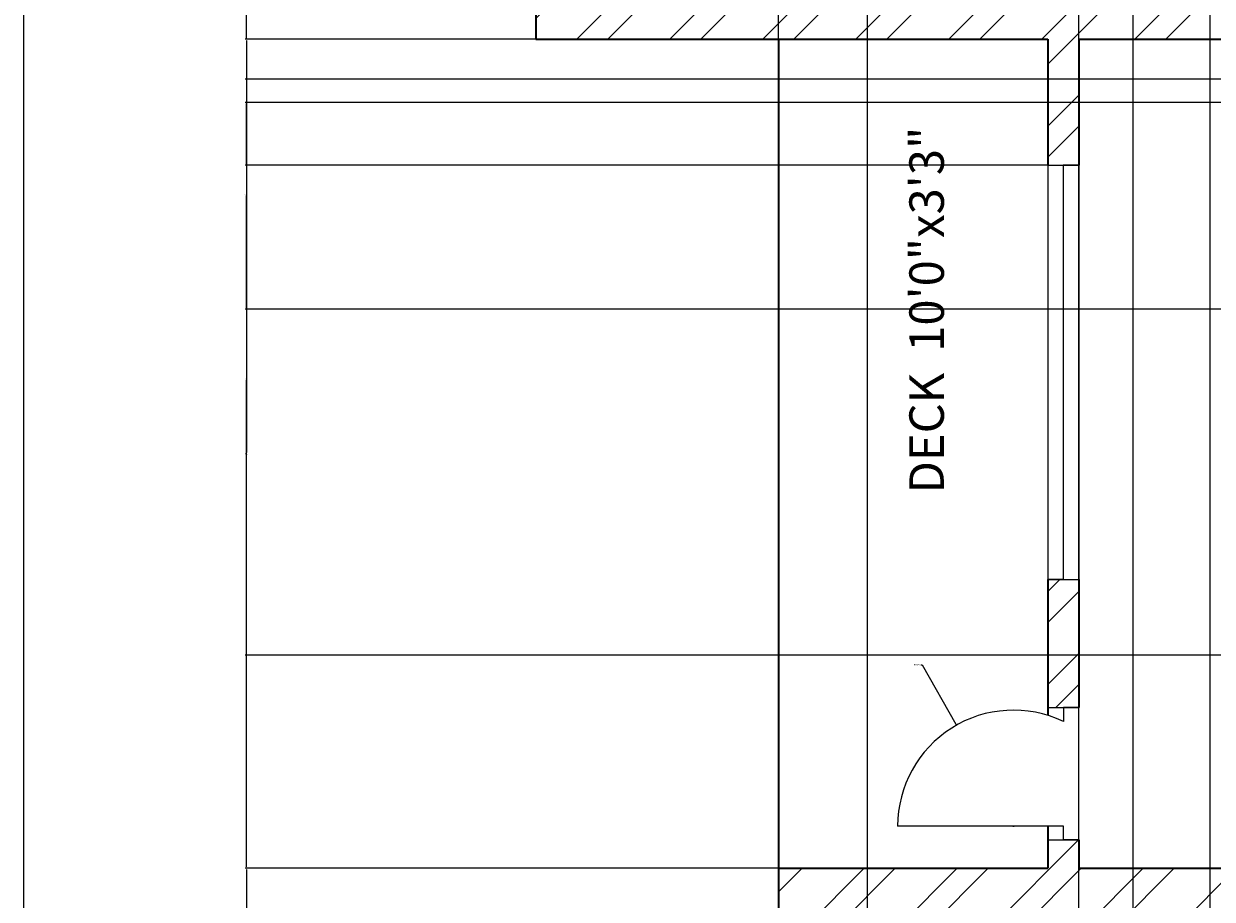
# Model space of a CAD drawing. Units: inches. Extents: x 1748 to 2382, y 1346 to 2284.
# Tile 7 of 26: x 1748 to 1920, y 1730 to 1857. Entities that reach past the tile are written whole.
import ezdxf

# ---------------------------------------------------------------- set-up
doc = ezdxf.new("R2010")
doc.units = ezdxf.units.IN
for name, color, linetype, lineweight in [('A-ANNO-DIMS', 2, 'Continuous', 18), ('A-ANNO-TTLB', 7, 'Continuous', 25), ('A-AREA-IDEN', 7, 'Continuous', 18), ('A-DOOR', 21, 'Continuous', 18), ('A-GLAZ', 191, 'Continuous', 18), ('A-WALL', 7, 'Continuous', 35), ('A-WALL-PATT', 9, 'Continuous', 13)]:
    doc.layers.add(name, color=color, linetype=linetype, lineweight=lineweight)
doc.styles.get("Standard").update_dxf_attribs({"font": 'arial.ttf'})
doc.dimstyles.get("Standard").update_dxf_attribs({"dimtxt": 0.18, "dimasz": 0.18, "dimexe": 0.18, "dimexo": 0.0625, "dimgap": 0.09, "dimtad": 0, "dimtih": 1, "dimtoh": 1, "dimdec": 4, "dimzin": 0, "dimdsep": 46, "dimtxsty": 'Standard', "dimcen": 0.09, "dimadec": 0, "dimazin": 0, "dimtfac": 1, "dimtdec": 4, "dimtofl": 0, "dimtmove": 0, "dimatfit": 3, "dimfxl": 1, "dimtolj": 1, "dimtzin": 0, "dimarcsym": 0})

# ---------------------------------------------------------------- blocks, each defined once
blk = doc.blocks.new('*D41')
at = {"layer": 'A-ANNO-DIMS', "color": 0, "lineweight": -2, "transparency": 16777216}
for p, q in [((1821.96, 1854.91), (1821.96, 2274.93)), ((1822.14, 2274.75), (1839.16, 2274.75)), ((1856.96, 2274.75), (1839.95, 2274.75)), ((1857.14, 1854.91), (1857.14, 2274.93))]:
    blk.add_line(p, q, dxfattribs=at)
at = {"layer": 'A-ANNO-DIMS', "color": 0, "transparency": 16777216}
for points in [[(1822.14, 2274.78), (1822.14, 2274.72), (1821.96, 2274.75)], [(1856.96, 2274.78), (1856.96, 2274.72), (1857.14, 2274.75)]]:
    blk.add_solid(points, dxfattribs=at)
at = {"layer": 'Defpoints', "color": 0, "transparency": 16777216}
for p in [(1857.14, 2274.75), (1821.96, 1854.85), (1857.14, 1854.85)]:
    blk.add_point(p, dxfattribs=at)
at = {"layer": 'A-ANNO-DIMS', "color": 0, "transparency": 16777216, "insert": (1839.55, 2274.75), "char_height": 0.18, "attachment_point": 5}
blk.add_mtext('\\A1;35.18', dxfattribs=at)
blk = doc.blocks.new('*D43')
at = {"layer": 'A-ANNO-DIMS', "color": 0, "lineweight": -2, "transparency": 16777216}
for p, q in [((1857.08, 1854.85), (1779.88, 1854.85)), ((1780.06, 1854.67), (1780.06, 1795.03)), ((1780.06, 1735.03), (1780.06, 1794.67)), ((1857.08, 1734.85), (1779.88, 1734.85))]:
    blk.add_line(p, q, dxfattribs=at)
at = {"layer": 'A-ANNO-DIMS', "color": 0, "transparency": 16777216}
for points in [[(1780.03, 1854.67), (1780.09, 1854.67), (1780.06, 1854.85)], [(1780.03, 1735.03), (1780.09, 1735.03), (1780.06, 1734.85)]]:
    blk.add_solid(points, dxfattribs=at)
at = {"layer": 'Defpoints', "color": 0, "transparency": 16777216}
for p in [(1780.06, 1854.85), (1857.14, 1854.85), (1857.14, 1734.85)]:
    blk.add_point(p, dxfattribs=at)
at = {"layer": 'A-ANNO-DIMS', "color": 0, "transparency": 16777216, "insert": (1780.06, 1794.85), "char_height": 0.18, "attachment_point": 5}
blk.add_mtext('\\A1;120', dxfattribs=at)
blk = doc.blocks.new('*D44')
at = {"layer": 'A-ANNO-DIMS', "color": 0, "lineweight": -2, "transparency": 16777216}
for p, q in [((1821.9, 1892.79), (1779.88, 1892.79)), ((1780.06, 1892.61), (1780.06, 1874)), ((1780.06, 1855.03), (1780.06, 1873.64)), ((1821.9, 1854.85), (1779.88, 1854.85))]:
    blk.add_line(p, q, dxfattribs=at)
at = {"layer": 'A-ANNO-DIMS', "color": 0, "transparency": 16777216}
for points in [[(1780.03, 1892.61), (1780.09, 1892.61), (1780.06, 1892.79)], [(1780.03, 1855.03), (1780.09, 1855.03), (1780.06, 1854.85)]]:
    blk.add_solid(points, dxfattribs=at)
at = {"layer": 'Defpoints', "color": 0, "transparency": 16777216}
for p in [(1780.06, 1892.79), (1821.96, 1892.79), (1821.96, 1854.85)]:
    blk.add_point(p, dxfattribs=at)
at = {"layer": 'A-ANNO-DIMS', "color": 0, "transparency": 16777216, "insert": (1780.06, 1873.82), "char_height": 0.18, "attachment_point": 5}
blk.add_mtext('\\A1;37.94', dxfattribs=at)
blk = doc.blocks.new('*D48')
at = {"layer": 'A-ANNO-DIMS', "color": 0, "lineweight": -2, "transparency": 16777216}
for p, q in [((2130.9, 1849.07), (1779.88, 1849.07)), ((1780.06, 1848.89), (1780.06, 1832.62)), ((1780.06, 1815.98), (1780.06, 1832.25)), ((2130.9, 1815.8), (1779.88, 1815.8))]:
    blk.add_line(p, q, dxfattribs=at)
at = {"layer": 'A-ANNO-DIMS', "color": 0, "transparency": 16777216}
for points in [[(1780.03, 1848.89), (1780.09, 1848.89), (1780.06, 1849.07)], [(1780.03, 1815.98), (1780.09, 1815.98), (1780.06, 1815.8)]]:
    blk.add_solid(points, dxfattribs=at)
at = {"layer": 'Defpoints', "color": 0, "transparency": 16777216}
for p in [(1780.06, 1849.07), (2130.96, 1849.07), (2130.96, 1815.8)]:
    blk.add_point(p, dxfattribs=at)
at = {"layer": 'A-ANNO-DIMS', "color": 0, "transparency": 16777216, "insert": (1780.06, 1832.43), "char_height": 0.18, "attachment_point": 5}
blk.add_mtext('\\A1;33.27', dxfattribs=at)
blk = doc.blocks.new('*D50')
at = {"layer": 'A-ANNO-DIMS', "color": 0, "lineweight": -2, "transparency": 16777216}
for p, q in [((1869.96, 2223.79), (1869.96, 1360.47)), ((1908.44, 2223.79), (1908.44, 1360.47)), ((1870.14, 1360.65), (1888.81, 1360.65)), ((1908.26, 1360.65), (1889.6, 1360.65))]:
    blk.add_line(p, q, dxfattribs=at)
at = {"layer": 'A-ANNO-DIMS', "color": 0, "transparency": 16777216}
for points in [[(1870.14, 1360.68), (1870.14, 1360.62), (1869.96, 1360.65)], [(1908.26, 1360.68), (1908.26, 1360.62), (1908.44, 1360.65)]]:
    blk.add_solid(points, dxfattribs=at)
at = {"layer": 'Defpoints', "color": 0, "transparency": 16777216}
for p in [(1869.96, 2223.85), (1908.44, 2223.85), (1908.44, 1360.65)]:
    blk.add_point(p, dxfattribs=at)
at = {"layer": 'A-ANNO-DIMS', "color": 0, "transparency": 16777216, "insert": (1889.2, 1360.65), "char_height": 0.18, "attachment_point": 5}
blk.add_mtext('\\A1;38.48', dxfattribs=at)
blk = doc.blocks.new('*D60')
at = {"layer": 'A-ANNO-DIMS', "color": 0, "lineweight": -2, "transparency": 16777216}
for p, q in [((2206.01, 1845.68), (1779.88, 1845.68)), ((1780.06, 1845.5), (1780.06, 1805.86)), ((1780.06, 1765.86), (1780.06, 1805.5)), ((2206.01, 1765.68), (1779.88, 1765.68))]:
    blk.add_line(p, q, dxfattribs=at)
at = {"layer": 'A-ANNO-DIMS', "color": 0, "transparency": 16777216}
for points in [[(1780.03, 1845.5), (1780.09, 1845.5), (1780.06, 1845.68)], [(1780.03, 1765.86), (1780.09, 1765.86), (1780.06, 1765.68)]]:
    blk.add_solid(points, dxfattribs=at)
at = {"layer": 'Defpoints', "color": 0, "transparency": 16777216}
for p in [(1780.06, 1845.68), (2206.07, 1845.68), (2206.07, 1765.68)]:
    blk.add_point(p, dxfattribs=at)
at = {"layer": 'A-ANNO-DIMS', "color": 0, "transparency": 16777216, "insert": (1780.06, 1805.68), "char_height": 0.18, "attachment_point": 5}
blk.add_mtext('\\A1;80', dxfattribs=at)
blk = doc.blocks.new('*D64')
at = {"layer": 'A-ANNO-DIMS', "color": 0, "lineweight": -2, "transparency": 16777216}
for p, q in [((1900.64, 1476.91), (1900.64, 2274.93)), ((1900.82, 2274.75), (1909.7, 2274.75)), ((1919.5, 2274.75), (1910.62, 2274.75)), ((1919.68, 1476.91), (1919.68, 2274.93))]:
    blk.add_line(p, q, dxfattribs=at)
at = {"layer": 'A-ANNO-DIMS', "color": 0, "transparency": 16777216}
for points in [[(1900.82, 2274.78), (1900.82, 2274.72), (1900.64, 2274.75)], [(1919.5, 2274.78), (1919.5, 2274.72), (1919.68, 2274.75)]]:
    blk.add_solid(points, dxfattribs=at)
at = {"layer": 'Defpoints', "color": 0, "transparency": 16777216}
for p in [(1919.68, 2274.75), (1900.64, 1476.85), (1919.68, 1476.85)]:
    blk.add_point(p, dxfattribs=at)
at = {"layer": 'A-ANNO-DIMS', "color": 0, "transparency": 16777216, "insert": (1910.16, 2274.75), "char_height": 0.18, "attachment_point": 5}
blk.add_mtext('\\A1;19.035', dxfattribs=at)
blk = doc.blocks.new('*D70')
at = {"layer": 'A-ANNO-DIMS', "color": 0, "lineweight": -2, "transparency": 16777216}
for p, q in [((1896.08, 1854.85), (1779.88, 1854.85)), ((1780.06, 1854.67), (1780.06, 1845.93)), ((1780.06, 1836.82), (1780.06, 1845.57)), ((1896.08, 1836.64), (1779.88, 1836.64))]:
    blk.add_line(p, q, dxfattribs=at)
at = {"layer": 'A-ANNO-DIMS', "color": 0, "transparency": 16777216}
for points in [[(1780.03, 1854.67), (1780.09, 1854.67), (1780.06, 1854.85)], [(1780.03, 1836.82), (1780.09, 1836.82), (1780.06, 1836.64)]]:
    blk.add_solid(points, dxfattribs=at)
at = {"layer": 'Defpoints', "color": 0, "transparency": 16777216}
for p in [(1780.06, 1854.85), (1896.14, 1854.85), (1896.14, 1836.64)]:
    blk.add_point(p, dxfattribs=at)
at = {"layer": 'A-ANNO-DIMS', "color": 0, "transparency": 16777216, "insert": (1780.06, 1845.75), "char_height": 0.18, "attachment_point": 5}
blk.add_mtext('\\A1;18.205', dxfattribs=at)
blk = doc.blocks.new('*D71')
at = {"layer": 'A-ANNO-DIMS', "color": 0, "lineweight": -2, "transparency": 16777216}
for p, q in [((1857.08, 1734.85), (1779.88, 1734.85)), ((1780.06, 1734.67), (1780.06, 1723.97)), ((1780.06, 1712.9), (1780.06, 1723.61)), ((1896.08, 1712.72), (1779.88, 1712.72))]:
    blk.add_line(p, q, dxfattribs=at)
at = {"layer": 'A-ANNO-DIMS', "color": 0, "transparency": 16777216}
for points in [[(1780.03, 1734.67), (1780.09, 1734.67), (1780.06, 1734.85)], [(1780.03, 1712.9), (1780.09, 1712.9), (1780.06, 1712.72)]]:
    blk.add_solid(points, dxfattribs=at)
at = {"layer": 'Defpoints', "color": 0, "transparency": 16777216}
for p in [(1780.06, 1734.85), (1857.14, 1734.85), (1896.14, 1712.72)]:
    blk.add_point(p, dxfattribs=at)
at = {"layer": 'A-ANNO-DIMS', "color": 0, "transparency": 16777216, "insert": (1780.06, 1723.79), "char_height": 0.18, "attachment_point": 5}
blk.add_mtext('\\A1;22.127', dxfattribs=at)
blk = doc.blocks.new('*D97')
at = {"layer": 'A-ANNO-DIMS', "color": 0, "lineweight": -2, "transparency": 16777216}
for p, q in [((1877.75, 1764.3), (1877.93, 1764.3)), ((1877.93, 1764.3), (1882.8, 1755.7)), ((1891.08, 1740.95), (1891.26, 1740.95)), ((1891.17, 1740.86), (1891.17, 1741.04))]:
    blk.add_line(p, q, dxfattribs=at)
at = {"layer": 'A-ANNO-DIMS', "color": 0, "transparency": 16777216}
blk.add_solid([(1882.83, 1755.71), (1882.78, 1755.68), (1882.89, 1755.54)], dxfattribs=at)
at = {"layer": 'Defpoints', "color": 0, "transparency": 16777216}
for p in [(1882.89, 1755.54), (1891.17, 1740.95)]:
    blk.add_point(p, dxfattribs=at)
at = {"layer": 'A-ANNO-DIMS', "color": 0, "transparency": 16777216, "insert": (1877.2, 1764.3), "char_height": 0.18, "attachment_point": 5}
blk.add_mtext('\\A1;R16.776', dxfattribs=at)

msp = doc.modelspace()

# ---------------------------------------------------------------- hatches: boundary and pattern name
at = {"layer": 'A-WALL-PATT'}
h = msp.add_hatch(dxfattribs=at)
h.set_pattern_fill('ANSI32', color=256)
h.paths.add_polyline_path([(1908.4445, 2232.8497), (1821.9607, 2232.8497), (1821.9607, 2223.8497), (1865.4607, 2223.8497), (1865.4607, 2209.9185), (1869.9607, 2209.9185), (1869.9607, 2223.8497), (1908.4445, 2223.8497), (1908.4445, 2228.3497)])
h.paths.add_polyline_path([(2040.0683, 2232.8497), (1968.4445, 2232.8497), (1968.4445, 2223.8497), (2025.9607, 2223.8497), (2025.9607, 2130.3497), (2032.1341, 2130.3497), (2032.1341, 2132.5997), (2032.1341, 2134.8497), (2030.4607, 2134.8497), (2030.4607, 2223.8497), (2040.0683, 2223.8497)])
h.paths.add_polyline_path([(2091.3969, 2232.8497), (2064.0683, 2232.8497), (2064.0683, 2223.8497), (2078.4607, 2223.8497), (2078.4607, 2134.8497), (2051.1563, 2134.8497), (2051.1563, 2130.3497), (2078.4607, 2130.3497), (2078.4607, 2128.6813), (2082.9607, 2128.6813), (2082.9607, 2130.3497), (2086.1879, 2130.3497), (2086.1879, 2132.5997), (2086.1879, 2134.8497), (2082.9607, 2134.8497), (2082.9607, 2223.8497), (2091.3969, 2223.8497), (2091.3969, 2228.3497)])
h.paths.add_polyline_path([(2167.0164, 2232.8497), (2115.3969, 2232.8497), (2115.3969, 2223.8497), (2130.9607, 2223.8497), (2130.9607, 2134.8497), (2106.9607, 2134.8497), (2106.9607, 2130.3497), (2135.4607, 2130.3497), (2135.4607, 2223.8497), (2167.0164, 2223.8497), (2167.0164, 2228.3497)])
h.paths.add_polyline_path([(1869.9607, 2149.9185), (1865.4607, 2149.9185), (1865.4607, 2127.8942), (1869.9607, 2127.8942)])
h.paths.add_polyline_path([(2082.9607, 2104.4871), (2080.7107, 2104.4871), (2078.4607, 2104.4871), (2078.4607, 2103.8497), (1869.9607, 2103.8497), (1869.9607, 2108.6062), (1867.7107, 2108.6062), (1865.4607, 2108.6062), (1865.4607, 2103.8497), (1821.9607, 2103.8497), (1821.9607, 2099.3497), (1865.4607, 2099.3497), (1865.4607, 2094.7509), (1869.9607, 2094.7509), (1869.9607, 2099.3497), (2025.9607, 2099.3497), (2025.9607, 2096.4326), (2030.4607, 2096.4326), (2030.4607, 2099.3497), (2082.9607, 2099.3497)])
h.paths.add_polyline_path([(1928.9457, 1401.1212), (2176.8693, 1401.1212), (2176.8693, 1438.214), (1928.9457, 1438.214)], flags=9)
h.paths.add_polyline_path([(2122.2668, 2048.1927), (2177.9387, 2048.1927), (2177.9387, 2066.85), (2122.2668, 2066.85)], flags=9)
h.paths.add_polyline_path([(2272.688, 2153.8197), (2272.688, 2216.746), (2262.3845, 2216.746), (2262.3845, 2153.8197)], flags=9)
h.paths.add_polyline_path([(2157.2928, 2166.5593), (2196.3822, 2166.5593), (2196.3822, 2185.2167), (2157.2928, 2185.2167)], flags=9)
h.paths.add_polyline_path([(2089.3407, 2162.0698), (2124.3987, 2162.0698), (2124.3987, 2180.7272), (2089.3407, 2180.7272)], flags=9)
h.paths.add_polyline_path([(2037.4521, 2160.0913), (2072.5101, 2160.0913), (2072.5101, 2178.7486), (2037.4521, 2178.7486)], flags=9)
h.paths.add_polyline_path([(1884.7894, 2104.1554), (1923.6297, 2104.1554), (1923.6297, 2122.8127), (1884.7894, 2122.8127)], flags=9)
h.paths.add_polyline_path([(1851.2832, 2142.9749), (1851.2832, 2199.3051), (1840.9796, 2199.3051), (1840.9796, 2142.9749)], flags=9)
h.paths.add_polyline_path([(1844.8763, 2017.2834), (1844.8763, 2073.6136), (1834.5728, 2073.6136), (1834.5728, 2017.2834)], flags=9)
h.paths.add_polyline_path([(1897.1577, 2073.1279), (1935.9981, 2073.1279), (1935.9981, 2091.7853), (1897.1577, 2091.7853)], flags=9)
h.paths.add_polyline_path([(1952.3395, 1802.4231), (2008.0114, 1802.4231), (2008.0114, 1821.0805), (1952.3395, 1821.0805)], flags=9)
h.paths.add_polyline_path([(1978.8184, 1857.6841), (2017.7338, 1857.6841), (2017.7338, 1876.3415), (1978.8184, 1876.3415)], flags=9)
h.paths.add_polyline_path([(1979.6513, 1925.9516), (2008.8089, 1925.9516), (2008.8089, 1944.6089), (1979.6513, 1944.6089)], flags=9)
h.paths.add_polyline_path([(1838.5553, 1860.3527), (1877.3957, 1860.3527), (1877.3957, 1879.01), (1838.5553, 1879.01)], flags=9)
h.paths.add_polyline_path([(1883.9018, 1787.3013), (1883.9018, 1843.6315), (1873.5983, 1843.6315), (1873.5983, 1787.3013)], flags=9)
h.paths.add_polyline_path([(1873.7079, 1509.1938), (1873.7079, 1583.7709), (1863.4044, 1583.7709), (1863.4044, 1509.1938)], flags=9)
h.paths.add_polyline_path([(1916.2259, 1603.3681), (1955.0663, 1603.3681), (1955.0663, 1622.0254), (1916.2259, 1622.0254)], flags=9)
h.paths.add_polyline_path([(1876.3013, 1636.757), (1876.3013, 1693.0871), (1865.9978, 1693.0871), (1865.9978, 1636.757)], flags=9)
h.paths.add_polyline_path([(1921.3138, 1521.8316), (1964.0662, 1521.8316), (1964.0662, 1540.489), (1921.3138, 1540.489)], flags=9)
h.paths.add_polyline_path([(2017.5657, 1497.5078), (2046.7983, 1497.5078), (2046.7983, 1516.1651), (2017.5657, 1516.1651)], flags=9)
h.paths.add_polyline_path([(2066.8661, 1499.3902), (2096.0988, 1499.3902), (2096.0988, 1518.0475), (2066.8661, 1518.0475)], flags=9)
h.paths.add_polyline_path([(2155.4835, 1571.6596), (2198.2358, 1571.6596), (2198.2358, 1590.3169), (2155.4835, 1590.3169)], flags=9)
h.paths.add_polyline_path([(2094.9136, 1664.6812), (2150.5855, 1664.6812), (2150.5855, 1683.3386), (2094.9136, 1683.3386)], flags=9)
h.paths.add_polyline_path([(2257.6902, 1863.1628), (2269.8935, 1863.1628), (2269.8935, 1873.4664), (2257.6902, 1873.4664)], flags=9)
h.paths.add_polyline_path([(2164.0748, 1880.3089), (2189.8694, 1880.3089), (2189.8694, 1890.6124), (2164.0748, 1890.6124)], flags=9)
h.paths.add_polyline_path([(2239.4394, 1931.0585), (2268.8187, 1931.0585), (2268.8187, 1949.7159), (2239.4394, 1949.7159)], flags=9)
h = msp.add_hatch(dxfattribs=at)
h.set_pattern_fill('ANSI32', color=256)
h.paths.add_polyline_path([(2297.4607, 2232.8497), (2203.0164, 2232.8497), (2203.0164, 2223.8497), (2244.9607, 2223.8497), (2244.9607, 2127.8554), (2249.4607, 2127.8554), (2249.4607, 2223.8497), (2297.4607, 2223.8497)])
h.paths.add_polyline_path([(2297.4607, 2103.8497), (2249.4607, 2103.8497), (2249.4607, 2106.7497), (2247.2107, 2106.7497), (2244.9607, 2106.7497), (2244.9607, 2103.8497), (2130.9607, 2103.8497), (2130.9607, 2099.3497), (2288.4607, 2099.3497), (2288.4607, 2077.2008), (2297.4607, 2077.2008)])
h.paths.add_polyline_path([(1928.9457, 1401.1212), (2176.8693, 1401.1212), (2176.8693, 1438.214), (1928.9457, 1438.214)], flags=9)
h.paths.add_polyline_path([(2122.2668, 2048.1927), (2177.9387, 2048.1927), (2177.9387, 2066.85), (2122.2668, 2066.85)], flags=9)
h.paths.add_polyline_path([(2272.688, 2153.8197), (2272.688, 2216.746), (2262.3845, 2216.746), (2262.3845, 2153.8197)], flags=25)
h.paths.add_polyline_path([(2157.2928, 2166.5593), (2196.3822, 2166.5593), (2196.3822, 2185.2167), (2157.2928, 2185.2167)], flags=9)
h.paths.add_polyline_path([(2089.3407, 2162.0698), (2124.3987, 2162.0698), (2124.3987, 2180.7272), (2089.3407, 2180.7272)], flags=9)
h.paths.add_polyline_path([(2037.4521, 2160.0913), (2072.5101, 2160.0913), (2072.5101, 2178.7486), (2037.4521, 2178.7486)], flags=9)
h.paths.add_polyline_path([(1884.7894, 2104.1554), (1923.6297, 2104.1554), (1923.6297, 2122.8127), (1884.7894, 2122.8127)], flags=9)
h.paths.add_polyline_path([(1851.2832, 2142.9749), (1851.2832, 2199.3051), (1840.9796, 2199.3051), (1840.9796, 2142.9749)], flags=9)
h.paths.add_polyline_path([(1844.8763, 2017.2834), (1844.8763, 2073.6136), (1834.5728, 2073.6136), (1834.5728, 2017.2834)], flags=9)
h.paths.add_polyline_path([(1897.1577, 2073.1279), (1935.9981, 2073.1279), (1935.9981, 2091.7853), (1897.1577, 2091.7853)], flags=9)
h.paths.add_polyline_path([(1952.3395, 1802.4231), (2008.0114, 1802.4231), (2008.0114, 1821.0805), (1952.3395, 1821.0805)], flags=9)
h.paths.add_polyline_path([(1978.8184, 1857.6841), (2017.7338, 1857.6841), (2017.7338, 1876.3415), (1978.8184, 1876.3415)], flags=9)
h.paths.add_polyline_path([(1979.6513, 1925.9516), (2008.8089, 1925.9516), (2008.8089, 1944.6089), (1979.6513, 1944.6089)], flags=9)
h.paths.add_polyline_path([(1838.5553, 1860.3527), (1877.3957, 1860.3527), (1877.3957, 1879.01), (1838.5553, 1879.01)], flags=9)
h.paths.add_polyline_path([(1883.9018, 1787.3013), (1883.9018, 1843.6315), (1873.5983, 1843.6315), (1873.5983, 1787.3013)], flags=9)
h.paths.add_polyline_path([(1873.7079, 1509.1938), (1873.7079, 1583.7709), (1863.4044, 1583.7709), (1863.4044, 1509.1938)], flags=9)
h.paths.add_polyline_path([(1916.2259, 1603.3681), (1955.0663, 1603.3681), (1955.0663, 1622.0254), (1916.2259, 1622.0254)], flags=9)
h.paths.add_polyline_path([(1876.3013, 1636.757), (1876.3013, 1693.0871), (1865.9978, 1693.0871), (1865.9978, 1636.757)], flags=9)
h.paths.add_polyline_path([(1921.3138, 1521.8316), (1964.0662, 1521.8316), (1964.0662, 1540.489), (1921.3138, 1540.489)], flags=9)
h.paths.add_polyline_path([(2017.5657, 1497.5078), (2046.7983, 1497.5078), (2046.7983, 1516.1651), (2017.5657, 1516.1651)], flags=9)
h.paths.add_polyline_path([(2066.8661, 1499.3902), (2096.0988, 1499.3902), (2096.0988, 1518.0475), (2066.8661, 1518.0475)], flags=9)
h.paths.add_polyline_path([(2155.4835, 1571.6596), (2198.2358, 1571.6596), (2198.2358, 1590.3169), (2155.4835, 1590.3169)], flags=9)
h.paths.add_polyline_path([(2094.9136, 1664.6812), (2150.5855, 1664.6812), (2150.5855, 1683.3386), (2094.9136, 1683.3386)], flags=9)
h.paths.add_polyline_path([(2257.6902, 1863.1628), (2269.8935, 1863.1628), (2269.8935, 1873.4664), (2257.6902, 1873.4664)], flags=9)
h.paths.add_polyline_path([(2164.0748, 1880.3089), (2189.8694, 1880.3089), (2189.8694, 1890.6124), (2164.0748, 1890.6124)], flags=9)
h.paths.add_polyline_path([(2239.4394, 1931.0585), (2268.8187, 1931.0585), (2268.8187, 1949.7159), (2239.4394, 1949.7159)], flags=9)
h = msp.add_hatch(dxfattribs=at)
h.set_pattern_fill('ANSI32', color=256)
h.paths.add_polyline_path([(1919.6777, 1476.8497), (1900.6426, 1476.8497), (1900.6426, 1522.0826), (1898.3926, 1522.0826), (1896.1426, 1522.0826), (1896.1426, 1476.8497), (1857.1426, 1476.8497), (1857.1426, 1467.8497), (1896.1426, 1467.8497), (1919.6777, 1467.8497), (1919.6777, 1472.3497)])
h.paths.add_polyline_path([(2018.7873, 1472.3497), (2018.7873, 1476.8497), (2010.9607, 1476.8497), (2010.9607, 1560.8497), (2034.9607, 1560.8497), (2034.9607, 1565.3497), (2006.4607, 1565.3497), (2006.4607, 1476.8497), (1955.6777, 1476.8497), (1955.6777, 1467.8497), (2018.7873, 1467.8497)])
h.paths.add_polyline_path([(2152.3354, 1472.3497), (2152.3354, 1476.8497), (2115.9607, 1476.8497), (2115.9607, 1565.3497), (2109.2204, 1565.3497), (2109.2204, 1563.0997), (2109.2204, 1560.8497), (2111.4607, 1560.8497), (2111.4607, 1476.8497), (2095.3617, 1476.8497), (2095.3617, 1467.8497), (2152.3354, 1467.8497)])
h.paths.add_polyline_path([(2071.3617, 1476.8497), (2063.4607, 1476.8497), (2063.4607, 1560.8497), (2090.1865, 1560.8497), (2090.1865, 1565.3497), (2063.4607, 1565.3497), (2063.4607, 1572.5485), (2061.2107, 1572.5485), (2058.9607, 1572.5485), (2058.9607, 1565.3497), (2055.6281, 1565.3497), (2055.6281, 1560.8497), (2058.9607, 1560.8497), (2058.9607, 1476.8497), (2042.7873, 1476.8497), (2042.7873, 1467.8497), (2071.3617, 1467.8497), (2071.3617, 1472.3497)])
h.paths.add_polyline_path([(2297.4607, 1506.5652), (2288.4607, 1506.5652), (2288.4607, 1476.8497), (2212.3354, 1476.8497), (2212.3354, 1467.8497), (2297.4607, 1467.8497)])
h.paths.add_polyline_path([(2297.4607, 1645.3038), (2288.4607, 1645.3038), (2288.4607, 1605.8497), (2058.9607, 1605.8497), (2058.9607, 1600.1857), (2061.2107, 1600.1857), (2063.4607, 1600.1857), (2063.4607, 1601.3497), (2288.4607, 1601.3497), (2288.4607, 1566.5652), (2297.4607, 1566.5652)])
h.paths.add_polyline_path([(2010.9607, 1609.0561), (2008.7107, 1609.0561), (2006.4607, 1609.0561), (2006.4607, 1605.8497), (1900.6426, 1605.8497), (1900.6426, 1609.7171), (1898.3926, 1609.7171), (1896.1426, 1609.7171), (1896.1426, 1605.8497), (1857.1426, 1605.8497), (1857.1426, 1601.3497), (1896.1426, 1601.3497), (1896.1426, 1542.5447), (1900.6426, 1542.5447), (1900.6426, 1601.3497), (2010.9607, 1601.3497)])
h.paths.add_polyline_path([(1928.9457, 1401.1212), (2176.8693, 1401.1212), (2176.8693, 1438.214), (1928.9457, 1438.214)], flags=9)
h.paths.add_polyline_path([(2122.2668, 2048.1927), (2177.9387, 2048.1927), (2177.9387, 2066.85), (2122.2668, 2066.85)], flags=9)
h.paths.add_polyline_path([(2272.688, 2153.8197), (2272.688, 2216.746), (2262.3845, 2216.746), (2262.3845, 2153.8197)], flags=9)
h.paths.add_polyline_path([(2157.2928, 2166.5593), (2196.3822, 2166.5593), (2196.3822, 2185.2167), (2157.2928, 2185.2167)], flags=9)
h.paths.add_polyline_path([(2089.3407, 2162.0698), (2124.3987, 2162.0698), (2124.3987, 2180.7272), (2089.3407, 2180.7272)], flags=9)
h.paths.add_polyline_path([(2037.4521, 2160.0913), (2072.5101, 2160.0913), (2072.5101, 2178.7486), (2037.4521, 2178.7486)], flags=9)
h.paths.add_polyline_path([(1884.7894, 2104.1554), (1923.6297, 2104.1554), (1923.6297, 2122.8127), (1884.7894, 2122.8127)], flags=9)
h.paths.add_polyline_path([(1851.2832, 2142.9749), (1851.2832, 2199.3051), (1840.9796, 2199.3051), (1840.9796, 2142.9749)], flags=9)
h.paths.add_polyline_path([(1844.8763, 2017.2834), (1844.8763, 2073.6136), (1834.5728, 2073.6136), (1834.5728, 2017.2834)], flags=9)
h.paths.add_polyline_path([(1897.1577, 2073.1279), (1935.9981, 2073.1279), (1935.9981, 2091.7853), (1897.1577, 2091.7853)], flags=9)
h.paths.add_polyline_path([(1952.3395, 1802.4231), (2008.0114, 1802.4231), (2008.0114, 1821.0805), (1952.3395, 1821.0805)], flags=9)
h.paths.add_polyline_path([(1978.8184, 1857.6841), (2017.7338, 1857.6841), (2017.7338, 1876.3415), (1978.8184, 1876.3415)], flags=9)
h.paths.add_polyline_path([(1979.6513, 1925.9516), (2008.8089, 1925.9516), (2008.8089, 1944.6089), (1979.6513, 1944.6089)], flags=9)
h.paths.add_polyline_path([(1838.5553, 1860.3527), (1877.3957, 1860.3527), (1877.3957, 1879.01), (1838.5553, 1879.01)], flags=9)
h.paths.add_polyline_path([(1883.9018, 1787.3013), (1883.9018, 1843.6315), (1873.5983, 1843.6315), (1873.5983, 1787.3013)], flags=9)
h.paths.add_polyline_path([(1873.7079, 1509.1938), (1873.7079, 1583.7709), (1863.4044, 1583.7709), (1863.4044, 1509.1938)], flags=9)
h.paths.add_polyline_path([(1916.2259, 1603.3681), (1955.0663, 1603.3681), (1955.0663, 1622.0254), (1916.2259, 1622.0254)], flags=9)
h.paths.add_polyline_path([(1876.3013, 1636.757), (1876.3013, 1693.0871), (1865.9978, 1693.0871), (1865.9978, 1636.757)], flags=9)
h.paths.add_polyline_path([(1921.3138, 1521.8316), (1964.0662, 1521.8316), (1964.0662, 1540.489), (1921.3138, 1540.489)], flags=9)
h.paths.add_polyline_path([(2017.5657, 1497.5078), (2046.7983, 1497.5078), (2046.7983, 1516.1651), (2017.5657, 1516.1651)], flags=9)
h.paths.add_polyline_path([(2066.8661, 1499.3902), (2096.0988, 1499.3902), (2096.0988, 1518.0475), (2066.8661, 1518.0475)], flags=9)
h.paths.add_polyline_path([(2155.4835, 1571.6596), (2198.2358, 1571.6596), (2198.2358, 1590.3169), (2155.4835, 1590.3169)], flags=25)
h.paths.add_polyline_path([(2094.9136, 1664.6812), (2150.5855, 1664.6812), (2150.5855, 1683.3386), (2094.9136, 1683.3386)], flags=9)
h.paths.add_polyline_path([(2257.6902, 1863.1628), (2269.8935, 1863.1628), (2269.8935, 1873.4664), (2257.6902, 1873.4664)], flags=9)
h.paths.add_polyline_path([(2164.0748, 1880.3089), (2189.8694, 1880.3089), (2189.8694, 1890.6124), (2164.0748, 1890.6124)], flags=9)
h.paths.add_polyline_path([(2239.4394, 1931.0585), (2268.8187, 1931.0585), (2268.8187, 1949.7159), (2239.4394, 1949.7159)], flags=9)
h = msp.add_hatch(dxfattribs=at)
h.set_pattern_fill('ANSI32', color=256)
h.paths.add_polyline_path([(1900.6426, 1652.723), (1896.1426, 1652.723), (1896.1426, 1629.9029), (1900.6426, 1629.9029)])
h.paths.add_polyline_path([(2206.0699, 1859.3497), (2197.0699, 1859.3497), (2197.0699, 1734.8497), (2206.0699, 1734.8497)], flags=17)
h.paths.add_polyline_path([(2297.4607, 1865.3269), (2288.4607, 1865.3269), (2288.4607, 1734.8497), (2206.0699, 1734.8497), (2180.4551, 1734.8497), (2180.4551, 1725.8497), (2197.0699, 1725.8497), (2206.0699, 1725.8497), (2288.4607, 1725.8497), (2288.4607, 1705.3038), (2297.4607, 1705.3038)])
h.paths.add_polyline_path([(2139.9607, 1815.8001), (2135.4607, 1815.8001), (2130.9607, 1815.8001), (2130.9607, 1734.8497), (1900.6426, 1734.8497), (1900.6426, 1738.9477), (1898.3926, 1738.9477), (1896.1426, 1738.9477), (1896.1426, 1734.8497), (1857.1426, 1734.8497), (1857.1426, 1725.8497), (1896.1426, 1725.8497), (1896.1426, 1712.723), (1900.6426, 1712.723), (1900.6426, 1725.8497), (2006.4607, 1725.8497), (2006.4607, 1637.448), (2010.9607, 1637.448), (2010.9607, 1725.8497), (2139.9607, 1725.8497), (2147.389, 1725.8497), (2147.389, 1730.3497), (2147.389, 1734.8497), (2139.9607, 1734.8497)])
h.paths.add_polyline_path([(2149.8497, 1917.8497), (2149.8497, 1922.3497), (2139.9607, 1922.3497), (2139.9607, 1979.3497), (2030.4607, 1979.3497), (2030.4607, 2069.8971), (2028.2107, 2069.8971), (2025.9607, 2069.8971), (2025.9607, 1979.3497), (1869.9607, 1979.3497), (1869.9607, 1998.93), (1865.4607, 1998.93), (1865.4607, 1979.3497), (1821.9607, 1979.3497), (1821.9607, 1952.7922), (1826.9306, 1952.7922), (1830.9607, 1952.7922), (1830.9607, 1970.3497), (1962.9607, 1970.3497), (1962.9607, 1926.5713), (1967.4607, 1926.5713), (1967.4607, 1970.3497), (2027.4607, 1970.3497), (2027.4607, 1898.3497), (2004.9604, 1898.3497), (2004.9604, 1893.8497), (2027.4607, 1893.8497), (2027.4607, 1859.3497), (1958.8973, 1859.3497), (1958.8973, 1854.8497), (2047.917, 1854.8497), (2047.917, 1859.3497), (2031.9607, 1859.3497), (2031.9607, 1970.3497), (2130.9607, 1970.3497), (2130.9607, 1859.3497), (2104.9565, 1859.3497), (2104.9565, 1854.8497), (2130.9607, 1854.8497), (2130.9607, 1849.0684), (2139.9607, 1849.0684), (2139.9607, 1913.3497), (2149.8497, 1913.3497)])
h.paths.add_polyline_path([(1928.9996, 1859.3497), (1830.9607, 1859.3497), (1830.9607, 1892.7922), (1821.9607, 1892.7922), (1821.9607, 1854.8497), (1896.1426, 1854.8497), (1896.1426, 1836.6443), (1898.378, 1836.6443), (1900.6426, 1836.6443), (1900.6426, 1854.8497), (1928.9996, 1854.8497), (1928.9996, 1857.0997)])
h.paths.add_polyline_path([(1980.9604, 1896.0997), (1980.9604, 1898.3497), (1967.4607, 1898.3497), (1967.4607, 1902.3846), (1962.9607, 1902.3846), (1962.9607, 1859.3497), (1967.4607, 1859.3497), (1967.4607, 1893.8497), (1980.9604, 1893.8497)], flags=17)
h.paths.add_polyline_path([(1900.6426, 1776.6443), (1896.1426, 1776.6443), (1896.1426, 1758.0891), (1900.6426, 1758.0891)], flags=17)
h.paths.add_polyline_path([(2297.4607, 2017.2008), (2288.4607, 2017.2008), (2288.4607, 1979.3497), (2213.4607, 1979.3497), (2213.4607, 1922.3497), (2183.3516, 1922.3497), (2183.3516, 1913.3497), (2213.4607, 1913.3497), (2236.234, 1913.3497), (2236.234, 1922.3497), (2222.4607, 1922.3497), (2222.4607, 1931.3497), (2222.4607, 1970.3497), (2288.4607, 1970.3497), (2288.4607, 1922.3497), (2272.1921, 1922.3497), (2272.1921, 1913.3497), (2288.4607, 1913.3497), (2288.4607, 1901.3269), (2297.4607, 1901.3269)])

# ---------------------------------------------------------------- linework, layer by layer
at = {"layer": 'A-ANNO-TTLB'}
msp.add_lwpolyline([(1747.8112, 2284.3704), (2382.1361, 2284.3704), (2382.1361, 1346.4899), (1747.8112, 1346.4899)], close=True, dxfattribs=at)
at = {"layer": 'A-DOOR'}
for p, q in [((1896.1426, 1758.0891), (1900.6426, 1758.0891)), ((1900.6426, 1758.0891), (1898.3926, 1758.0891)), ((1898.3926, 1758.0891), (1898.3926, 1756.0891)), ((1898.3926, 1740.9477), (1874.3926, 1740.9477)), ((1898.3926, 1738.9477), (1898.3926, 1740.9477)), ((1896.1426, 1738.9477), (1900.6426, 1738.9477)), ((1900.6426, 1738.9477), (1898.3926, 1738.9477))]:
    msp.add_line(p, q, dxfattribs=at)
msp.add_arc((1891.1689, 1740.9477), 16.7763, 64.49492, 180, dxfattribs=at)
at = {"layer": 'A-GLAZ'}
for p, q in [((1896.1426, 1836.6443), (1898.378, 1836.6443)), ((1896.1426, 1836.6443), (1896.1426, 1776.6443)), ((1898.378, 1836.6443), (1900.6426, 1836.6443)), ((1900.6426, 1836.6443), (1898.378, 1836.6443)), ((1898.378, 1836.6443), (1898.378, 1776.6443)), ((1900.6426, 1836.6443), (1900.6426, 1776.6443)), ((1898.378, 1776.6443), (1896.1426, 1776.6443)), ((1896.1426, 1776.6443), (1900.6426, 1776.6443))]:
    msp.add_line(p, q, dxfattribs=at)
at = {"layer": 'A-WALL'}
for p, q in [((1821.9607, 1892.7922), (1821.9607, 1854.8497)), ((1821.9607, 1854.8497), (1896.1426, 1854.8497)), ((1857.1426, 1854.8497), (1857.1426, 1605.8497)), ((1896.1426, 1854.8497), (1896.1426, 1836.6443)), ((1900.6426, 1854.8497), (1900.6426, 1836.6443)), ((1900.6426, 1854.8497), (1928.9996, 1854.8497)), ((1896.1426, 1776.6443), (1896.1426, 1756.9697)), ((1900.6426, 1776.6443), (1900.6426, 1758.0891)), ((1896.1426, 1740.9477), (1896.1426, 1734.8497)), ((1900.6426, 1738.9477), (1900.6426, 1734.8497)), ((1857.1426, 1734.8497), (1896.1426, 1734.8497)), ((1900.6426, 1734.8497), (2130.9607, 1734.8497))]:
    msp.add_line(p, q, dxfattribs=at)

# ---------------------------------------------------------------- texts
at = {"layer": 'A-AREA-IDEN', "insert": (1876.0863, 1789.0902), "char_height": 5, "attachment_point": 1, "rotation": 90}
msp.add_mtext_dynamic_manual_height_columns('DECK  10\'0"x3\'3"', width=286.800511, gutter_width=12.5, heights=[0], dxfattribs=at)

# ---------------------------------------------------------------- dimensions: what is measured, and where the dimension line sits
at = {"layer": 'A-ANNO-DIMS'}
for base, p1, p2, override, picture, middle in [((1857.1426, 2274.7497), (1821.9607, 1854.8497), (1857.1426, 1854.8497), {"dimdec": 2, "dimlfac": 1, "dimrnd": 0, "dimzin": 0, "dimdsep": 46, "dimlunit": 2}, '*D41', (1839.5517, 2274.7497)), ((1919.6777, 2274.7497), (1900.6426, 1476.8497), (1919.6777, 1476.8497), {"dimdec": 3, "dimlfac": 1, "dimrnd": 0, "dimzin": 0, "dimdsep": 46, "dimlunit": 2}, '*D64', (1910.1602, 2274.7497)), ((1908.4445, 1360.6451), (1869.9607, 2223.8497), (1908.4445, 2223.8497), {"dimdec": 2, "dimlfac": 1, "dimrnd": 0, "dimzin": 0, "dimdsep": 46, "dimlunit": 2}, '*D50', (1889.2026, 1360.6451))]:
    dim = msp.add_linear_dim(base=base, p1=p1, p2=p2, dimstyle='Standard', override=override, dxfattribs=at)
    dim.commit()
    dim.dimension.update_dxf_attribs({"geometry": picture, "text_midpoint": middle})
for base, p1, p2, override, picture, middle in [((1780.0607, 1892.7922), (1821.9607, 1854.8497), (1821.9607, 1892.7922), {"dimdec": 2, "dimlfac": 1, "dimrnd": 0, "dimzin": 0, "dimdsep": 46, "dimlunit": 2}, '*D44', (1780.0607, 1873.8209)), ((1780.0607, 1854.8497), (1896.1426, 1836.6443), (1896.1426, 1854.8497), {"dimdec": 3, "dimlfac": 1, "dimrnd": 0, "dimzin": 0, "dimdsep": 46, "dimlunit": 2}, '*D70', (1780.0607, 1845.747)), ((1780.0607, 1854.8497), (1857.1426, 1734.8497), (1857.1426, 1854.8497), {"dimdec": 0, "dimlfac": 1, "dimrnd": 0, "dimzin": 0, "dimdsep": 46, "dimlunit": 2}, '*D43', (1780.0607, 1794.8497)), ((1780.0607, 1849.0684), (2130.9607, 1815.8001), (2130.9607, 1849.0684), {"dimdec": 2, "dimlfac": 1, "dimrnd": 0, "dimzin": 0, "dimdsep": 46, "dimlunit": 2}, '*D48', (1780.0607, 1832.4343)), ((1780.0607, 1845.6799), (2206.0699, 1765.6799), (2206.0699, 1845.6799), {"dimdec": 0, "dimlfac": 1, "dimrnd": 0, "dimzin": 0, "dimdsep": 46, "dimlunit": 2}, '*D60', (1780.0607, 1805.6799)), ((1780.0607, 1734.8497), (1896.1426, 1712.723), (1857.1426, 1734.8497), {"dimdec": 3, "dimlfac": 1, "dimrnd": 0, "dimzin": 0, "dimdsep": 46, "dimlunit": 2}, '*D71', (1780.0607, 1723.7863))]:
    dim = msp.add_linear_dim(base=base, p1=p1, p2=p2, angle=90, dimstyle='Standard', override=override, dxfattribs=at)
    dim.commit()
    dim.dimension.update_dxf_attribs({"geometry": picture, "text_midpoint": middle})
dim = msp.add_radius_dim(center=(1891.1689, 1740.9477), mpoint=(1882.8933, 1755.5408), dimstyle='Standard', override={"dimdec": 3, "dimlfac": 1, "dimrnd": 0, "dimzin": 0, "dimdsep": 46, "dimlunit": 2}, dxfattribs=at)
dim.commit()
dim.dimension.update_dxf_attribs({"geometry": '*D97', "text_midpoint": (1877.1983, 1764.2966), "dimtype": 164})

doc.saveas('drawing.dxf')
